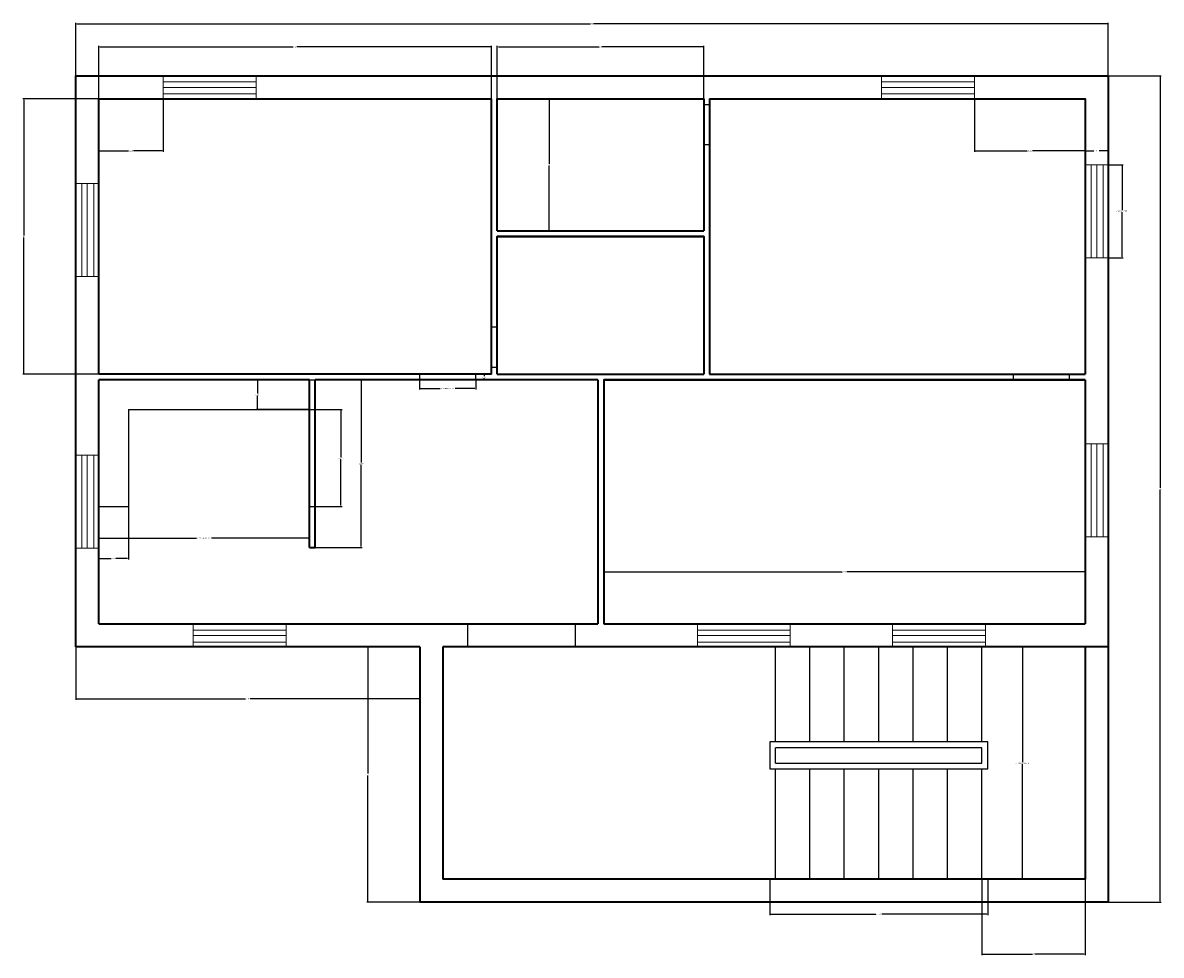
# Model space of a CAD drawing. Units: feet. Extents: x 1914 to 2338, y 2098 to 2528.
# Tile 1 of 3: x 1914 to 2112, y 2098 to 2260. Entities that reach past the tile are written whole.
import ezdxf

# ---------------------------------------------------------------- set-up
doc = ezdxf.new("R2010")
doc.units = ezdxf.units.FT
for name, color, linetype, lineweight in [('A-ANNO-DIMS', 2, 'Continuous', 18), ('A-DOOR', 3, 'Continuous', 25), ('A-FLOR-CASE', 8, 'Continuous', 25), ('A-FLOR-STRS', 7, 'Continuous', 25), ('A-GLAZ', 4, 'Continuous', 18), ('A-WALL', 7, 'Continuous', 35)]:
    doc.layers.add(name, color=color, linetype=linetype, lineweight=lineweight)
doc.styles.get("Standard").update_dxf_attribs({"font": 'arial.ttf'})
doc.dimstyles.get("Standard").update_dxf_attribs({"dimtxt": 0.18, "dimasz": 0.18, "dimexe": 0.18, "dimexo": 0.0625, "dimgap": 0.09, "dimtad": 0, "dimtih": 1, "dimtoh": 1, "dimdec": 1, "dimzin": 0, "dimdsep": 46, "dimlunit": 3, "dimtxsty": 'Standard', "dimcen": 0.09, "dimadec": 0, "dimazin": 0, "dimtfac": 1, "dimtdec": 1, "dimtofl": 0, "dimtmove": 0, "dimatfit": 3, "dimfxl": 1, "dimtolj": 1, "dimtzin": 0, "dimarcsym": 0})

# ---------------------------------------------------------------- blocks, each defined once
blk = doc.blocks.new('WIN-PLAN')
for p, q in [((0, 0), (0, 4)), ((16.2, 4), (16.2, 0)), ((16.2, 2.93), (0, 2.93)), ((16.2, 1.98), (0, 1.98)), ((16.2, 0.84), (0, 0.84))]:
    blk.add_line(p, q)
blk = doc.blocks.new('WIN-PLAN-OUTER-EDGE')
for p, q in [((0, 0), (0, 4)), ((0, 4), (16.2, 4)), ((16.2, 4), (16.2, 0)), ((16.2, 2.93), (0, 2.93)), ((16.2, 1.98), (0, 1.98)), ((16.2, 0.84), (0, 0.84))]:
    blk.add_line(p, q)
blk.add_lwpolyline([(0, 4), (16.2, 4)])
blk = doc.blocks.new('STAIR-RETURN-FLIGHT')
for p, q in [((1, 23.92), (1, 40.5)), ((7, 23.92), (7, 40.5)), ((13, 23.92), (13, 40.5)), ((19, 23.92), (19, 40.5)), ((25, 23.92), (25, 40.5)), ((31, 23.92), (31, 40.5)), ((37, 23.92), (37, 40.5)), ((1, 20.25), (1, 22.92)), ((37, 20.25), (37, 22.92)), ((1, 0), (1, 19.25)), ((7, 0), (7, 19.25)), ((13, 0), (13, 19.25)), ((19, 0), (19, 19.25)), ((25, 0), (25, 19.25)), ((31, 0), (31, 19.25)), ((37, 0), (37, 19.25))]:
    blk.add_line(p, q)
blk.add_lwpolyline([(0, 19.25), (38, 19.25), (38, 23.92), (0, 23.92)], close=True)
for points in [[(37, 22.92), (1, 22.92)], [(1, 20.25), (37, 20.25)]]:
    blk.add_lwpolyline(points)
blk = doc.blocks.new('COUNTER-L')
for p, q in [((5.19, 16.93), (5.19, 0)), ((5.19, 16.93), (36.73, 16.93)), ((0, 0), (5.19, 0))]:
    blk.add_line(p, q)
blk = doc.blocks.new('OPENING-ENTRY')
for points in [[(0, 4), (0, 0)], [(18.83, 0), (18.83, 4)]]:
    blk.add_lwpolyline(points)
blk = doc.blocks.new('OPENING-INTERIOR-WIDE')
blk.add_lwpolyline([(9.8, 0), (9.8, 1), (0, 1), (0, 0)], close=True)
blk = doc.blocks.new('OPENING-INTERIOR-NARROW')
blk.add_lwpolyline([(0, 7.05), (1, 7.05), (1, 0), (0, 0)], close=True)
blk = doc.blocks.new('*D8')
at = {"layer": 'A-ANNO-DIMS', "color": 0, "lineweight": -2, "transparency": 16777216}
for p, q in [((2102.91, 2235.34), (2105.46, 2235.34)), ((2105.28, 2235.16), (2105.28, 2227.43)), ((2105.28, 2219.32), (2105.28, 2227.06)), ((2102.91, 2219.14), (2105.46, 2219.14))]:
    blk.add_line(p, q, dxfattribs=at)
at = {"layer": 'A-ANNO-DIMS', "color": 0, "transparency": 16777216}
for points in [[(2105.25, 2235.16), (2105.31, 2235.16), (2105.28, 2235.34)], [(2105.25, 2219.32), (2105.31, 2219.32), (2105.28, 2219.14)]]:
    blk.add_solid(points, dxfattribs=at)
at = {"layer": 'Defpoints', "color": 0, "transparency": 16777216}
for p in [(2102.85, 2235.34), (2105.28, 2235.34), (2102.85, 2219.14)]:
    blk.add_point(p, dxfattribs=at)
at = {"layer": 'A-ANNO-DIMS', "color": 0, "transparency": 16777216, "insert": (2105.28, 2227.24), "char_height": 0.18, "attachment_point": 5}
blk.add_mtext('\\A1;WINDOW 16 TYP.', dxfattribs=at)
blk = doc.blocks.new('*D9')
at = {"layer": 'A-ANNO-DIMS', "color": 0, "lineweight": -2, "transparency": 16777216}
for p, q in [((2098.85, 2235.41), (2098.85, 2237.95)), ((2099.03, 2237.77), (2100.38, 2237.77)), ((2102.67, 2237.77), (2101.31, 2237.77)), ((2102.85, 2235.41), (2102.85, 2237.95))]:
    blk.add_line(p, q, dxfattribs=at)
at = {"layer": 'A-ANNO-DIMS', "color": 0, "transparency": 16777216}
for points in [[(2099.03, 2237.8), (2099.03, 2237.74), (2098.85, 2237.77)], [(2102.67, 2237.8), (2102.67, 2237.74), (2102.85, 2237.77)]]:
    blk.add_solid(points, dxfattribs=at)
at = {"layer": 'Defpoints', "color": 0, "transparency": 16777216}
for p in [(2098.85, 2237.77), (2098.85, 2235.34), (2102.85, 2235.34)]:
    blk.add_point(p, dxfattribs=at)
at = {"layer": 'A-ANNO-DIMS', "color": 0, "transparency": 16777216, "insert": (2100.85, 2237.77), "char_height": 0.18, "attachment_point": 5}
blk.add_mtext('\\A1;4 TYP.', dxfattribs=at)
blk = doc.blocks.new('*D12')
at = {"layer": 'A-ANNO-DIMS', "color": 0, "lineweight": -2, "transparency": 16777216}
for p, q in [((1982.79, 2197.79), (1982.79, 2196.2)), ((1992.59, 2197.79), (1992.59, 2196.2)), ((1982.97, 2196.38), (1986.38, 2196.38)), ((1992.41, 2196.38), (1989, 2196.38))]:
    blk.add_line(p, q, dxfattribs=at)
at = {"layer": 'A-ANNO-DIMS', "color": 0, "transparency": 16777216}
for points in [[(1982.97, 2196.41), (1982.97, 2196.35), (1982.79, 2196.38)], [(1992.41, 2196.41), (1992.41, 2196.35), (1992.59, 2196.38)]]:
    blk.add_solid(points, dxfattribs=at)
at = {"layer": 'Defpoints', "color": 0, "transparency": 16777216}
for p in [(1982.79, 2197.85), (1992.59, 2197.85), (1992.59, 2196.38)]:
    blk.add_point(p, dxfattribs=at)
at = {"layer": 'A-ANNO-DIMS', "color": 0, "transparency": 16777216, "insert": (1987.69, 2196.38), "char_height": 0.18, "attachment_point": 5}
blk.add_mtext('\\A1;WIDE DOOR 10 TYP.', dxfattribs=at)
blk = doc.blocks.new('*D13')
at = {"layer": 'A-ANNO-DIMS', "color": 0, "lineweight": -2, "transparency": 16777216}
for p, q in [((1992.65, 2198.85), (1994.24, 2198.85)), ((1992.65, 2197.85), (1994.24, 2197.85)), ((1994.06, 2198.67), (1994.06, 2198.53)), ((1994.06, 2198.03), (1994.06, 2198.17))]:
    blk.add_line(p, q, dxfattribs=at)
at = {"layer": 'A-ANNO-DIMS', "color": 0, "transparency": 16777216}
for points in [[(1994.03, 2198.67), (1994.09, 2198.67), (1994.06, 2198.85)], [(1994.03, 2198.03), (1994.09, 2198.03), (1994.06, 2197.85)]]:
    blk.add_solid(points, dxfattribs=at)
at = {"layer": 'Defpoints', "color": 0, "transparency": 16777216}
for p in [(1992.59, 2198.85), (1992.59, 2197.85), (1994.06, 2198.85)]:
    blk.add_point(p, dxfattribs=at)
at = {"layer": 'A-ANNO-DIMS', "color": 0, "transparency": 16777216, "insert": (1994.06, 2198.35), "char_height": 0.18, "attachment_point": 5}
blk.add_mtext('\\A1;1 TYP.', dxfattribs=at)
blk = doc.blocks.new('*D18')
at = {"layer": 'A-ANNO-DIMS', "color": 0, "lineweight": -2, "transparency": 16777216}
for p, q in [((2081.91, 2151.35), (2088.1, 2151.35)), ((2087.92, 2151.17), (2087.92, 2131.28)), ((2087.92, 2111.03), (2087.92, 2130.92)), ((2081.91, 2110.85), (2088.1, 2110.85))]:
    blk.add_line(p, q, dxfattribs=at)
at = {"layer": 'A-ANNO-DIMS', "color": 0, "transparency": 16777216}
for points in [[(2087.89, 2151.17), (2087.95, 2151.17), (2087.92, 2151.35)], [(2087.89, 2111.03), (2087.95, 2111.03), (2087.92, 2110.85)]]:
    blk.add_solid(points, dxfattribs=at)
at = {"layer": 'Defpoints', "color": 0, "transparency": 16777216}
for p in [(2081.85, 2151.35), (2087.92, 2151.35), (2081.85, 2110.85)]:
    blk.add_point(p, dxfattribs=at)
at = {"layer": 'A-ANNO-DIMS', "color": 0, "transparency": 16777216, "insert": (2087.92, 2131.1), "char_height": 0.18, "attachment_point": 5}
blk.add_mtext('\\A1;RETURN STAIR 41 TYP.', dxfattribs=at)
blk = doc.blocks.new('*D19')
at = {"layer": 'A-ANNO-DIMS', "color": 0, "lineweight": -2, "transparency": 16777216}
for p, q in [((2043.85, 2110.79), (2043.85, 2104.59)), ((2081.85, 2110.79), (2081.85, 2104.59)), ((2044.03, 2104.77), (2062.32, 2104.77)), ((2081.67, 2104.77), (2063.37, 2104.77))]:
    blk.add_line(p, q, dxfattribs=at)
at = {"layer": 'A-ANNO-DIMS', "color": 0, "transparency": 16777216}
for points in [[(2044.03, 2104.8), (2044.03, 2104.74), (2043.85, 2104.77)], [(2081.67, 2104.8), (2081.67, 2104.74), (2081.85, 2104.77)]]:
    blk.add_solid(points, dxfattribs=at)
at = {"layer": 'Defpoints', "color": 0, "transparency": 16777216}
for p in [(2043.85, 2110.85), (2081.85, 2110.85), (2081.85, 2104.77)]:
    blk.add_point(p, dxfattribs=at)
at = {"layer": 'A-ANNO-DIMS', "color": 0, "transparency": 16777216, "insert": (2062.85, 2104.77), "char_height": 0.18, "attachment_point": 5}
blk.add_mtext('\\A1;38 TYP.', dxfattribs=at)
blk = doc.blocks.new('*D20')
at = {"layer": 'A-ANNO-DIMS', "color": 0, "lineweight": -2, "transparency": 16777216}
for p, q in [((1926.85, 2175.72), (1926.85, 2170.09)), ((1963.58, 2175.72), (1963.58, 2170.09)), ((1927.03, 2170.27), (1943.92, 2170.27)), ((1963.4, 2170.27), (1946.5, 2170.27))]:
    blk.add_line(p, q, dxfattribs=at)
at = {"layer": 'A-ANNO-DIMS', "color": 0, "transparency": 16777216}
for points in [[(1927.03, 2170.3), (1927.03, 2170.24), (1926.85, 2170.27)], [(1963.4, 2170.3), (1963.4, 2170.24), (1963.58, 2170.27)]]:
    blk.add_solid(points, dxfattribs=at)
at = {"layer": 'Defpoints', "color": 0, "transparency": 16777216}
for p in [(1926.85, 2175.78), (1963.58, 2175.78), (1963.58, 2170.27)]:
    blk.add_point(p, dxfattribs=at)
at = {"layer": 'A-ANNO-DIMS', "color": 0, "transparency": 16777216, "insert": (1945.21, 2170.27), "char_height": 0.18, "attachment_point": 5}
blk.add_mtext('\\A1;L-COUNTER 37 TYP.', dxfattribs=at)
blk = doc.blocks.new('*D21')
at = {"layer": 'A-ANNO-DIMS', "color": 0, "lineweight": -2, "transparency": 16777216}
for p, q in [((1963.64, 2192.71), (1969.27, 2192.71)), ((1969.09, 2192.53), (1969.09, 2184.42)), ((1969.09, 2175.96), (1969.09, 2184.06)), ((1963.64, 2175.78), (1969.27, 2175.78))]:
    blk.add_line(p, q, dxfattribs=at)
at = {"layer": 'A-ANNO-DIMS', "color": 0, "transparency": 16777216}
for points in [[(1969.06, 2192.53), (1969.12, 2192.53), (1969.09, 2192.71)], [(1969.06, 2175.96), (1969.12, 2175.96), (1969.09, 2175.78)]]:
    blk.add_solid(points, dxfattribs=at)
at = {"layer": 'Defpoints', "color": 0, "transparency": 16777216}
for p in [(1963.58, 2192.71), (1969.09, 2192.71), (1963.58, 2175.78)]:
    blk.add_point(p, dxfattribs=at)
at = {"layer": 'A-ANNO-DIMS', "color": 0, "transparency": 16777216, "insert": (1969.09, 2184.24), "char_height": 0.18, "attachment_point": 5}
blk.add_mtext('\\A1;17 TYP.', dxfattribs=at)
blk = doc.blocks.new('*D22')
at = {"layer": 'A-ANNO-DIMS', "color": 0, "lineweight": -2, "transparency": 16777216}
for p, q in [((1922.85, 2250.91), (1922.85, 2260.08)), ((1923.03, 2259.9), (2012.57, 2259.9)), ((2102.67, 2259.9), (2013.13, 2259.9)), ((2102.85, 2250.91), (2102.85, 2260.08))]:
    blk.add_line(p, q, dxfattribs=at)
at = {"layer": 'A-ANNO-DIMS', "color": 0, "transparency": 16777216}
for points in [[(1923.03, 2259.93), (1923.03, 2259.87), (1922.85, 2259.9)], [(2102.67, 2259.93), (2102.67, 2259.87), (2102.85, 2259.9)]]:
    blk.add_solid(points, dxfattribs=at)
at = {"layer": 'Defpoints', "color": 0, "transparency": 16777216}
for p in [(2102.85, 2259.9), (1922.85, 2250.85), (2102.85, 2250.85)]:
    blk.add_point(p, dxfattribs=at)
at = {"layer": 'A-ANNO-DIMS', "color": 0, "transparency": 16777216, "insert": (2012.85, 2259.9), "char_height": 0.18, "attachment_point": 5}
blk.add_mtext('\\A1;180', dxfattribs=at)
blk = doc.blocks.new('*D23')
at = {"layer": 'A-ANNO-DIMS', "color": 0, "lineweight": -2, "transparency": 16777216}
for p, q in [((2102.91, 2250.85), (2112.08, 2250.85)), ((2111.9, 2250.67), (2111.9, 2179.03)), ((2111.9, 2107.03), (2111.9, 2178.67)), ((2102.91, 2106.85), (2112.08, 2106.85))]:
    blk.add_line(p, q, dxfattribs=at)
at = {"layer": 'A-ANNO-DIMS', "color": 0, "transparency": 16777216}
for points in [[(2111.87, 2250.67), (2111.93, 2250.67), (2111.9, 2250.85)], [(2111.87, 2107.03), (2111.93, 2107.03), (2111.9, 2106.85)]]:
    blk.add_solid(points, dxfattribs=at)
at = {"layer": 'Defpoints', "color": 0, "transparency": 16777216}
for p in [(2102.85, 2250.85), (2111.9, 2250.85), (2102.85, 2106.85)]:
    blk.add_point(p, dxfattribs=at)
at = {"layer": 'A-ANNO-DIMS', "color": 0, "transparency": 16777216, "insert": (2111.9, 2178.85), "char_height": 0.18, "attachment_point": 5}
blk.add_mtext('\\A1;144', dxfattribs=at)
blk = doc.blocks.new('*D24')
at = {"layer": 'A-ANNO-DIMS', "color": 0, "lineweight": -2, "transparency": 16777216}
for p, q in [((1922.85, 2151.29), (1922.85, 2142.11)), ((1982.83, 2151.29), (1982.83, 2142.11)), ((1923.03, 2142.29), (1952.44, 2142.29)), ((1982.65, 2142.29), (1953.23, 2142.29))]:
    blk.add_line(p, q, dxfattribs=at)
at = {"layer": 'A-ANNO-DIMS', "color": 0, "transparency": 16777216}
for points in [[(1923.03, 2142.32), (1923.03, 2142.26), (1922.85, 2142.29)], [(1982.65, 2142.32), (1982.65, 2142.26), (1982.83, 2142.29)]]:
    blk.add_solid(points, dxfattribs=at)
at = {"layer": 'Defpoints', "color": 0, "transparency": 16777216}
for p in [(1922.85, 2151.35), (1982.83, 2151.35), (1922.85, 2142.29)]:
    blk.add_point(p, dxfattribs=at)
at = {"layer": 'A-ANNO-DIMS', "color": 0, "transparency": 16777216, "insert": (1952.84, 2142.29), "char_height": 0.18, "attachment_point": 5}
blk.add_mtext('\\A1;59.98', dxfattribs=at)
blk = doc.blocks.new('*D25')
at = {"layer": 'A-ANNO-DIMS', "color": 0, "lineweight": -2, "transparency": 16777216}
for p, q in [((1982.77, 2151.35), (1973.59, 2151.35)), ((1973.77, 2151.17), (1973.77, 2129.28)), ((1973.77, 2107.03), (1973.77, 2128.92)), ((1982.77, 2106.85), (1973.59, 2106.85))]:
    blk.add_line(p, q, dxfattribs=at)
at = {"layer": 'A-ANNO-DIMS', "color": 0, "transparency": 16777216}
for points in [[(1973.74, 2151.17), (1973.8, 2151.17), (1973.77, 2151.35)], [(1973.74, 2107.03), (1973.8, 2107.03), (1973.77, 2106.85)]]:
    blk.add_solid(points, dxfattribs=at)
at = {"layer": 'Defpoints', "color": 0, "transparency": 16777216}
for p in [(1973.77, 2151.35), (1982.83, 2151.35), (1982.83, 2106.85)]:
    blk.add_point(p, dxfattribs=at)
at = {"layer": 'A-ANNO-DIMS', "color": 0, "transparency": 16777216, "insert": (1973.77, 2129.1), "char_height": 0.18, "attachment_point": 5}
blk.add_mtext('\\A1;44.5', dxfattribs=at)
blk = doc.blocks.new('*D26')
at = {"layer": 'A-ANNO-DIMS', "color": 0, "lineweight": -2, "transparency": 16777216}
for p, q in [((1926.85, 2246.91), (1926.85, 2256.08)), ((1927.03, 2255.9), (1960.77, 2255.9)), ((1995.17, 2255.9), (1961.42, 2255.9)), ((1995.35, 2246.91), (1995.35, 2256.08))]:
    blk.add_line(p, q, dxfattribs=at)
at = {"layer": 'A-ANNO-DIMS', "color": 0, "transparency": 16777216}
for points in [[(1927.03, 2255.93), (1927.03, 2255.87), (1926.85, 2255.9)], [(1995.17, 2255.93), (1995.17, 2255.87), (1995.35, 2255.9)]]:
    blk.add_solid(points, dxfattribs=at)
at = {"layer": 'Defpoints', "color": 0, "transparency": 16777216}
for p in [(1995.35, 2255.9), (1926.85, 2246.85), (1995.35, 2246.85)]:
    blk.add_point(p, dxfattribs=at)
at = {"layer": 'A-ANNO-DIMS', "color": 0, "transparency": 16777216, "insert": (1961.1, 2255.9), "char_height": 0.18, "attachment_point": 5}
blk.add_mtext('\\A1;68.5', dxfattribs=at)
blk = doc.blocks.new('*D27')
at = {"layer": 'A-ANNO-DIMS', "color": 0, "lineweight": -2, "transparency": 16777216}
for p, q in [((1996.35, 2246.91), (1996.35, 2256.08)), ((1996.53, 2255.9), (2014.13, 2255.9)), ((2032.17, 2255.9), (2014.56, 2255.9)), ((2032.35, 2246.91), (2032.35, 2256.08))]:
    blk.add_line(p, q, dxfattribs=at)
at = {"layer": 'A-ANNO-DIMS', "color": 0, "transparency": 16777216}
for points in [[(1996.53, 2255.93), (1996.53, 2255.87), (1996.35, 2255.9)], [(2032.17, 2255.93), (2032.17, 2255.87), (2032.35, 2255.9)]]:
    blk.add_solid(points, dxfattribs=at)
at = {"layer": 'Defpoints', "color": 0, "transparency": 16777216}
for p in [(2032.35, 2255.9), (1996.35, 2246.85), (2032.35, 2246.85)]:
    blk.add_point(p, dxfattribs=at)
at = {"layer": 'A-ANNO-DIMS', "color": 0, "transparency": 16777216, "insert": (2014.35, 2255.9), "char_height": 0.18, "attachment_point": 5}
blk.add_mtext('\\A1;36', dxfattribs=at)
blk = doc.blocks.new('*D28')
at = {"layer": 'A-ANNO-DIMS', "color": 0, "lineweight": -2, "transparency": 16777216}
for p, q in [((1926.78, 2246.85), (1913.61, 2246.85)), ((1913.79, 2246.67), (1913.79, 2223.03)), ((1913.79, 2199.03), (1913.79, 2222.67)), ((1926.78, 2198.85), (1913.61, 2198.85))]:
    blk.add_line(p, q, dxfattribs=at)
at = {"layer": 'A-ANNO-DIMS', "color": 0, "transparency": 16777216}
for points in [[(1913.76, 2246.67), (1913.82, 2246.67), (1913.79, 2246.85)], [(1913.76, 2199.03), (1913.82, 2199.03), (1913.79, 2198.85)]]:
    blk.add_solid(points, dxfattribs=at)
at = {"layer": 'Defpoints', "color": 0, "transparency": 16777216}
for p in [(1913.79, 2246.85), (1926.85, 2246.85), (1926.85, 2198.85)]:
    blk.add_point(p, dxfattribs=at)
at = {"layer": 'A-ANNO-DIMS', "color": 0, "transparency": 16777216, "insert": (1913.79, 2222.85), "char_height": 0.18, "attachment_point": 5}
blk.add_mtext('\\A1;48', dxfattribs=at)
blk = doc.blocks.new('*D29')
at = {"layer": 'A-ANNO-DIMS', "color": 0, "lineweight": -2, "transparency": 16777216}
for p, q in [((1996.41, 2246.85), (2005.58, 2246.85)), ((2005.4, 2246.67), (2005.4, 2235.53)), ((2005.4, 2224.03), (2005.4, 2235.17)), ((1996.41, 2223.85), (2005.58, 2223.85))]:
    blk.add_line(p, q, dxfattribs=at)
at = {"layer": 'A-ANNO-DIMS', "color": 0, "transparency": 16777216}
for points in [[(2005.37, 2246.67), (2005.43, 2246.67), (2005.4, 2246.85)], [(2005.37, 2224.03), (2005.43, 2224.03), (2005.4, 2223.85)]]:
    blk.add_solid(points, dxfattribs=at)
at = {"layer": 'Defpoints', "color": 0, "transparency": 16777216}
for p in [(1996.35, 2246.85), (1996.35, 2223.85), (2005.4, 2223.85)]:
    blk.add_point(p, dxfattribs=at)
at = {"layer": 'A-ANNO-DIMS', "color": 0, "transparency": 16777216, "insert": (2005.4, 2235.35), "char_height": 0.18, "attachment_point": 5}
blk.add_mtext('\\A1;23', dxfattribs=at)
blk = doc.blocks.new('*D30')
at = {"layer": 'A-ANNO-DIMS', "color": 0, "lineweight": -2, "transparency": 16777216}
for p, q in [((2014.9, 2155.41), (2014.9, 2164.58)), ((2015.08, 2164.4), (2056.48, 2164.4)), ((2098.67, 2164.4), (2057.27, 2164.4)), ((2098.85, 2155.41), (2098.85, 2164.58))]:
    blk.add_line(p, q, dxfattribs=at)
at = {"layer": 'A-ANNO-DIMS', "color": 0, "transparency": 16777216}
for points in [[(2015.08, 2164.43), (2015.08, 2164.37), (2014.9, 2164.4)], [(2098.67, 2164.43), (2098.67, 2164.37), (2098.85, 2164.4)]]:
    blk.add_solid(points, dxfattribs=at)
at = {"layer": 'Defpoints', "color": 0, "transparency": 16777216}
for p in [(2098.85, 2164.4), (2014.9, 2155.35), (2098.85, 2155.35)]:
    blk.add_point(p, dxfattribs=at)
at = {"layer": 'A-ANNO-DIMS', "color": 0, "transparency": 16777216, "insert": (2056.87, 2164.4), "char_height": 0.18, "attachment_point": 5}
blk.add_mtext('\\A1;83.95', dxfattribs=at)
blk = doc.blocks.new('*D31')
at = {"layer": 'A-ANNO-DIMS', "color": 0, "lineweight": -2, "transparency": 16777216}
for p, q in [((1963.64, 2197.85), (1972.81, 2197.85)), ((1972.63, 2197.67), (1972.63, 2183.44)), ((1972.63, 2168.85), (1972.63, 2183.08)), ((1963.64, 2168.67), (1972.81, 2168.67))]:
    blk.add_line(p, q, dxfattribs=at)
at = {"layer": 'A-ANNO-DIMS', "color": 0, "transparency": 16777216}
for points in [[(1972.6, 2197.67), (1972.66, 2197.67), (1972.63, 2197.85)], [(1972.6, 2168.85), (1972.66, 2168.85), (1972.63, 2168.67)]]:
    blk.add_solid(points, dxfattribs=at)
at = {"layer": 'Defpoints', "color": 0, "transparency": 16777216}
for p in [(1963.58, 2197.85), (1963.58, 2168.67), (1972.63, 2168.67)]:
    blk.add_point(p, dxfattribs=at)
at = {"layer": 'A-ANNO-DIMS', "color": 0, "transparency": 16777216, "insert": (1972.63, 2183.26), "char_height": 0.18, "attachment_point": 5}
blk.add_mtext('\\A1;29.177', dxfattribs=at)
blk = doc.blocks.new('*D32')
at = {"layer": 'A-ANNO-DIMS', "color": 0, "lineweight": -2, "transparency": 16777216}
for p, q in [((1926.85, 2175.72), (1926.85, 2166.54)), ((1932.04, 2175.72), (1932.04, 2166.54)), ((1927.03, 2166.72), (1929.05, 2166.72)), ((1931.86, 2166.72), (1929.83, 2166.72))]:
    blk.add_line(p, q, dxfattribs=at)
at = {"layer": 'A-ANNO-DIMS', "color": 0, "transparency": 16777216}
for points in [[(1927.03, 2166.75), (1927.03, 2166.69), (1926.85, 2166.72)], [(1931.86, 2166.75), (1931.86, 2166.69), (1932.04, 2166.72)]]:
    blk.add_solid(points, dxfattribs=at)
at = {"layer": 'Defpoints', "color": 0, "transparency": 16777216}
for p in [(1926.85, 2175.78), (1932.04, 2175.78), (1926.85, 2166.72)]:
    blk.add_point(p, dxfattribs=at)
at = {"layer": 'A-ANNO-DIMS', "color": 0, "transparency": 16777216, "insert": (1929.44, 2166.72), "char_height": 0.18, "attachment_point": 5}
blk.add_mtext('\\A1;5.189', dxfattribs=at)
blk = doc.blocks.new('*D33')
at = {"layer": 'A-ANNO-DIMS', "color": 0, "lineweight": -2, "transparency": 16777216}
for p, q in [((1963.52, 2197.85), (1954.34, 2197.85)), ((1954.52, 2197.67), (1954.52, 2195.46)), ((1954.52, 2192.89), (1954.52, 2195.1)), ((1963.52, 2192.71), (1954.34, 2192.71))]:
    blk.add_line(p, q, dxfattribs=at)
at = {"layer": 'A-ANNO-DIMS', "color": 0, "transparency": 16777216}
for points in [[(1954.49, 2197.67), (1954.55, 2197.67), (1954.52, 2197.85)], [(1954.49, 2192.89), (1954.55, 2192.89), (1954.52, 2192.71)]]:
    blk.add_solid(points, dxfattribs=at)
at = {"layer": 'Defpoints', "color": 0, "transparency": 16777216}
for p in [(1954.52, 2197.85), (1963.58, 2197.85), (1963.58, 2192.71)]:
    blk.add_point(p, dxfattribs=at)
at = {"layer": 'A-ANNO-DIMS', "color": 0, "transparency": 16777216, "insert": (1954.52, 2195.28), "char_height": 0.18, "attachment_point": 5}
blk.add_mtext('\\A1;5.143', dxfattribs=at)
blk = doc.blocks.new('*D34')
at = {"layer": 'A-ANNO-DIMS', "color": 0, "lineweight": -2, "transparency": 16777216}
for p, q in [((2080.85, 2110.79), (2080.85, 2097.61)), ((2098.85, 2110.79), (2098.85, 2097.61)), ((2081.03, 2097.79), (2089.64, 2097.79)), ((2098.67, 2097.79), (2090.06, 2097.79))]:
    blk.add_line(p, q, dxfattribs=at)
at = {"layer": 'A-ANNO-DIMS', "color": 0, "transparency": 16777216}
for points in [[(2081.03, 2097.82), (2081.03, 2097.76), (2080.85, 2097.79)], [(2098.67, 2097.82), (2098.67, 2097.76), (2098.85, 2097.79)]]:
    blk.add_solid(points, dxfattribs=at)
at = {"layer": 'Defpoints', "color": 0, "transparency": 16777216}
for p in [(2080.85, 2110.85), (2098.85, 2110.85), (2080.85, 2097.79)]:
    blk.add_point(p, dxfattribs=at)
at = {"layer": 'A-ANNO-DIMS', "color": 0, "transparency": 16777216, "insert": (2089.85, 2097.79), "char_height": 0.18, "attachment_point": 5}
blk.add_mtext('\\A1;18', dxfattribs=at)
blk = doc.blocks.new('*D40')
at = {"layer": 'A-ANNO-DIMS', "color": 0, "lineweight": -2, "transparency": 16777216}
for p, q in [((1926.85, 2246.79), (1926.85, 2237.61)), ((1938.1, 2246.79), (1938.1, 2237.61)), ((1927.03, 2237.79), (1932.02, 2237.79)), ((1937.92, 2237.79), (1932.93, 2237.79))]:
    blk.add_line(p, q, dxfattribs=at)
at = {"layer": 'A-ANNO-DIMS', "color": 0, "transparency": 16777216}
for points in [[(1927.03, 2237.82), (1927.03, 2237.76), (1926.85, 2237.79)], [(1937.92, 2237.82), (1937.92, 2237.76), (1938.1, 2237.79)]]:
    blk.add_solid(points, dxfattribs=at)
at = {"layer": 'Defpoints', "color": 0, "transparency": 16777216}
for p in [(1926.85, 2246.85), (1938.1, 2246.85), (1926.85, 2237.79)]:
    blk.add_point(p, dxfattribs=at)
at = {"layer": 'A-ANNO-DIMS', "color": 0, "transparency": 16777216, "insert": (1932.47, 2237.79), "char_height": 0.18, "attachment_point": 5}
blk.add_mtext('\\A1;11.258', dxfattribs=at)
blk = doc.blocks.new('*D41')
at = {"layer": 'A-ANNO-DIMS', "color": 0, "lineweight": -2, "transparency": 16777216}
for p, q in [((2079.55, 2246.79), (2079.55, 2237.61)), ((2098.85, 2246.79), (2098.85, 2237.61)), ((2079.73, 2237.79), (2088.75, 2237.79)), ((2098.67, 2237.79), (2089.65, 2237.79))]:
    blk.add_line(p, q, dxfattribs=at)
at = {"layer": 'A-ANNO-DIMS', "color": 0, "transparency": 16777216}
for points in [[(2079.73, 2237.82), (2079.73, 2237.76), (2079.55, 2237.79)], [(2098.67, 2237.82), (2098.67, 2237.76), (2098.85, 2237.79)]]:
    blk.add_solid(points, dxfattribs=at)
at = {"layer": 'Defpoints', "color": 0, "transparency": 16777216}
for p in [(2079.55, 2246.85), (2098.85, 2246.85), (2079.55, 2237.79)]:
    blk.add_point(p, dxfattribs=at)
at = {"layer": 'A-ANNO-DIMS', "color": 0, "transparency": 16777216, "insert": (2089.2, 2237.79), "char_height": 0.18, "attachment_point": 5}
blk.add_mtext('\\A1;19.292', dxfattribs=at)

msp = doc.modelspace()

# ---------------------------------------------------------------- linework, layer by layer
at = {"layer": 'A-WALL'}
for p, q in [((2013.8999, 2197.8486), (1996.0126, 2197.8486)), ((1996.3458, 2198.8486), (2032.3458, 2198.8486)), ((2013.8999, 2197.8486), (2013.8999, 2155.3486)), ((2014.8458, 2197.8486), (2098.8458, 2197.8486)), ((2098.8458, 2197.8486), (2014.8999, 2197.8486)), ((2014.8999, 2197.8486), (2014.8999, 2155.3486)), ((2033.3458, 2198.8486), (2098.8458, 2198.8486)), ((1963.5782, 2168.6719), (1964.5782, 2168.6719)), ((1986.8289, 2155.3486), (2013.8999, 2155.3486)), ((2014.8999, 2155.3486), (2098.8458, 2155.3486)), ((2098.8458, 2151.3486), (2086.8458, 2151.3486)), ((1982.8289, 2110.8486), (1982.8289, 2106.8486))]:
    msp.add_line(p, q, dxfattribs=at)
for points in [[(1922.8458, 2151.3486), (1922.8458, 2250.8486), (2102.8458, 2250.8486), (2102.8458, 2106.8486), (1982.8289, 2106.8486)], [(1926.8458, 2198.8486), (1926.8458, 2246.8486), (1995.3458, 2246.8486)], [(1995.3458, 2198.8486), (1995.3458, 2246.8486)], [(1996.3458, 2246.8486), (2032.3458, 2246.8486)], [(1996.3458, 2223.8486), (1996.3458, 2246.8486)], [(2032.3458, 2246.8486), (2032.3458, 2223.8486)], [(2033.3458, 2246.8486), (2033.3458, 2198.8486)], [(2033.3458, 2246.8486), (2098.8458, 2246.8486), (2098.8458, 2198.8486)], [(1996.3458, 2223.8486), (2032.3458, 2223.8486)], [(2032.3458, 2222.8486), (1996.3458, 2222.8486)], [(1996.3458, 2198.8486), (1996.3458, 2222.8486), (2032.3458, 2222.8486), (2032.3458, 2198.8486)], [(1995.3458, 2198.8486), (1926.8458, 2198.8486)], [(1926.8458, 2155.3486), (1926.8458, 2197.8486)], [(1963.5782, 2197.8486), (1926.8458, 2197.8486)], [(1963.5782, 2168.6719), (1963.5782, 2197.8486)], [(2013.8999, 2197.8486), (1964.5782, 2197.8486)], [(1964.5782, 2168.6719), (1964.5782, 2197.8486)], [(2098.8458, 2197.8486), (2098.8458, 2155.3486)], [(1926.8458, 2155.3486), (1986.8289, 2155.3486)], [(1982.8289, 2151.3486), (1922.8458, 2151.3486)], [(1982.8289, 2151.3486), (1982.8289, 2110.8486)], [(1986.8289, 2151.3486), (1986.8289, 2110.8486)], [(2098.8458, 2151.3486), (2098.8458, 2110.8486), (1986.8289, 2110.8486)], [(2102.8458, 2151.3486), (1986.8289, 2151.3486)]]:
    msp.add_lwpolyline(points, dxfattribs=at)

# ---------------------------------------------------------------- block references
at = {"layer": 'A-DOOR'}
for name, p in [('OPENING-INTERIOR-NARROW', (2032.3458, 2238.7895)), ('OPENING-INTERIOR-NARROW', (1995.3458, 2200.0275)), ('OPENING-INTERIOR-WIDE', (1982.7892, 2197.8486)), ('OPENING-INTERIOR-WIDE', (2086.2892, 2197.8486)), ('OPENING-ENTRY', (1991.1775, 2151.3486))]:
    msp.add_blockref(name, p, dxfattribs=at)
at = {"layer": 'A-FLOR-CASE'}
msp.add_blockref('COUNTER-L', (1926.8458, 2175.7782), dxfattribs=at)
at = {"layer": 'A-FLOR-STRS'}
msp.add_blockref('STAIR-RETURN-FLIGHT', (2043.8458, 2110.8486), dxfattribs=at)
at = {"layer": 'A-GLAZ'}
for name, p in [('WIN-PLAN-OUTER-EDGE', (1938.1038, 2246.8486)), ('WIN-PLAN', (2063.3543, 2246.8486)), ('WIN-PLAN', (1943.3321, 2151.3486)), ('WIN-PLAN', (2031.2272, 2151.3486)), ('WIN-PLAN', (2065.2754, 2151.3486))]:
    msp.add_blockref(name, p, dxfattribs=at)
for p, rotation in [((2102.8458, 2219.144), 90.00000000000684), ((1926.8458, 2215.9), 90.00000000000225), ((2102.8458, 2170.5134), 90.00000000000757), ((1926.8458, 2168.565), 90.00000000000306)]:
    msp.add_blockref('WIN-PLAN', p, dxfattribs=dict(at, rotation=rotation))

# ---------------------------------------------------------------- dimensions: what is measured, and where the dimension line sits
at = {"layer": 'A-ANNO-DIMS'}
for base, p1, p2, override, picture, middle in [((2102.8458, 2259.9036), (1922.8458, 2250.8486), (2102.8458, 2250.8486), {"dimdec": 0, "dimlfac": 1, "dimrnd": 0, "dimzin": 0, "dimdsep": 46, "dimlunit": 2}, '*D22', (2012.8458, 2259.9036)), ((1995.3458, 2255.9036), (1926.8458, 2246.8486), (1995.3458, 2246.8486), {"dimdec": 1, "dimlfac": 1, "dimrnd": 0, "dimzin": 0, "dimdsep": 46, "dimlunit": 2}, '*D26', (1961.0958, 2255.9036)), ((2032.3458, 2255.9036), (1996.3458, 2246.8486), (2032.3458, 2246.8486), {"dimdec": 0, "dimlfac": 1, "dimrnd": 0, "dimzin": 0, "dimdsep": 46, "dimlunit": 2}, '*D27', (2014.3458, 2255.9036)), ((2098.8458, 2164.4036), (2014.8999, 2155.3486), (2098.8458, 2155.3486), {"dimdec": 2, "dimlfac": 1, "dimrnd": 0, "dimzin": 0, "dimdsep": 46, "dimlunit": 2}, '*D30', (2056.8728, 2164.4036)), ((2080.8458, 2097.7936), (2098.8458, 2110.8486), (2080.8458, 2110.8486), {"dimdec": 0, "dimlfac": 1, "dimrnd": 0, "dimzin": 0, "dimdsep": 46, "dimlunit": 2}, '*D34', (2089.8458, 2097.7936))]:
    dim = msp.add_linear_dim(base=base, p1=p1, p2=p2, dimstyle='Standard', override=override, dxfattribs=at)
    dim.commit()
    dim.dimension.update_dxf_attribs({"geometry": picture, "text_midpoint": middle})
for base, p1, p2, angle, override, picture, middle in [((2111.9008, 2250.8486), (2102.8458, 2106.8486), (2102.8458, 2250.8486), 90, {"dimdec": 0, "dimlfac": 1, "dimrnd": 0, "dimzin": 0, "dimdsep": 46, "dimlunit": 2}, '*D23', (2111.9008, 2178.8486)), ((1913.7908, 2246.8486), (1926.8458, 2198.8486), (1926.8458, 2246.8486), 90, {"dimdec": 0, "dimlfac": 1, "dimrnd": 0, "dimzin": 0, "dimdsep": 46, "dimlunit": 2}, '*D28', (1913.7908, 2222.8486)), ((1926.8458, 2237.7936), (1938.1038, 2246.8486), (1926.8458, 2246.8486), 180, {"dimdec": 3, "dimlfac": 1, "dimrnd": 0, "dimzin": 0, "dimdsep": 46, "dimlunit": 2}, '*D40', (1932.4748, 2237.7936)), ((2005.4008, 2223.8486), (1996.3458, 2246.8486), (1996.3458, 2223.8486), 270, {"dimdec": 0, "dimlfac": 1, "dimrnd": 0, "dimzin": 0, "dimdsep": 46, "dimlunit": 2}, '*D29', (2005.4008, 2235.3486)), ((2079.5536, 2237.7936), (2098.8458, 2246.8486), (2079.5536, 2246.8486), 180, {"dimdec": 3, "dimlfac": 1, "dimrnd": 0, "dimzin": 0, "dimdsep": 46, "dimlunit": 2}, '*D41', (2089.1997, 2237.7936)), ((1954.5232, 2197.8486), (1963.5782, 2192.7057), (1963.5782, 2197.8486), 90, {"dimdec": 3, "dimlfac": 1, "dimrnd": 0, "dimzin": 0, "dimdsep": 46, "dimlunit": 2}, '*D33', (1954.5232, 2195.2772)), ((1972.6332, 2168.6719), (1963.5782, 2197.8486), (1963.5782, 2168.6719), 270, {"dimdec": 3, "dimlfac": 1, "dimrnd": 0, "dimzin": 0, "dimdsep": 46, "dimlunit": 2}, '*D31', (1972.6332, 2183.2603)), ((1926.84582, 2166.7232), (1932.03529, 2175.7782), (1926.84582, 2175.7782), 180, {"dimdec": 3, "dimlfac": 1, "dimrnd": 0, "dimzin": 0, "dimdsep": 46, "dimlunit": 2}, '*D32', (1929.44056, 2166.7232)), ((1922.8458, 2142.2936), (1982.8289, 2151.3486), (1922.8458, 2151.3486), 180, {"dimdec": 2, "dimlfac": 1, "dimrnd": 0, "dimzin": 0, "dimdsep": 46, "dimlunit": 2}, '*D24', (1952.8374, 2142.2936)), ((1973.7739, 2151.3486), (1982.8289, 2106.8486), (1982.8289, 2151.3486), 90, {"dimdec": 1, "dimlfac": 1, "dimrnd": 0, "dimzin": 0, "dimdsep": 46, "dimlunit": 2}, '*D25', (1973.7739, 2129.0986))]:
    dim = msp.add_linear_dim(base=base, p1=p1, p2=p2, angle=angle, dimstyle='Standard', override=override, dxfattribs=at)
    dim.commit()
    dim.dimension.update_dxf_attribs({"geometry": picture, "text_midpoint": middle})
for base, p1, p2, angle, text, picture, middle in [((2098.8458, 2237.7731), (2102.8458, 2235.3432), (2098.8458, 2235.3432), 180, '<> TYP.', '*D9', (2100.8458, 2237.7731)), ((2105.2757, 2235.3432), (2102.8458, 2219.144), (2102.8458, 2235.3432), 90, 'WINDOW <> TYP.', '*D8', (2105.2757, 2227.2436)), ((1994.0573, 2198.8486), (1992.5875, 2197.8486), (1992.5875, 2198.8486), 90, '<> TYP.', '*D13', (1994.0573, 2198.3486)), ((1969.088, 2192.7057), (1963.5782, 2175.7782), (1963.5782, 2192.7057), 90, '<> TYP.', '*D21', (1969.088, 2184.242)), ((2087.9208213805, 2151.3485968592), (2081.8458213805, 2110.8485968592), (2081.8458213805, 2151.3485968592), 90, 'RETURN STAIR <> TYP.', '*D18', (2087.9208213805, 2131.0985968592))]:
    dim = msp.add_linear_dim(base=base, p1=p1, p2=p2, angle=angle, text=text, dimstyle='Standard', override={"dimdec": 0, "dimlfac": 1, "dimrnd": 0, "dimzin": 0, "dimdsep": 46, "dimlunit": 2}, dxfattribs=at)
    dim.commit()
    dim.dimension.update_dxf_attribs({"geometry": picture, "text_midpoint": middle})
for base, p1, p2, text, picture, middle in [((1992.5875, 2196.3788), (1982.7892, 2197.8486), (1992.5875, 2197.8486), 'WIDE DOOR <> TYP.', '*D12', (1987.6884, 2196.3788)), ((1963.5782, 2170.2683), (1926.8458, 2175.7782), (1963.5782, 2175.7782), 'L-COUNTER <> TYP.', '*D20', (1945.212, 2170.2683)), ((2081.8458, 2104.7736), (2043.8458, 2110.8486), (2081.8458, 2110.8486), '<> TYP.', '*D19', (2062.8458, 2104.7736))]:
    dim = msp.add_linear_dim(base=base, p1=p1, p2=p2, text=text, dimstyle='Standard', override={"dimdec": 0, "dimlfac": 1, "dimrnd": 0, "dimzin": 0, "dimdsep": 46, "dimlunit": 2}, dxfattribs=at)
    dim.commit()
    dim.dimension.update_dxf_attribs({"geometry": picture, "text_midpoint": middle})

doc.saveas('drawing.dxf')
